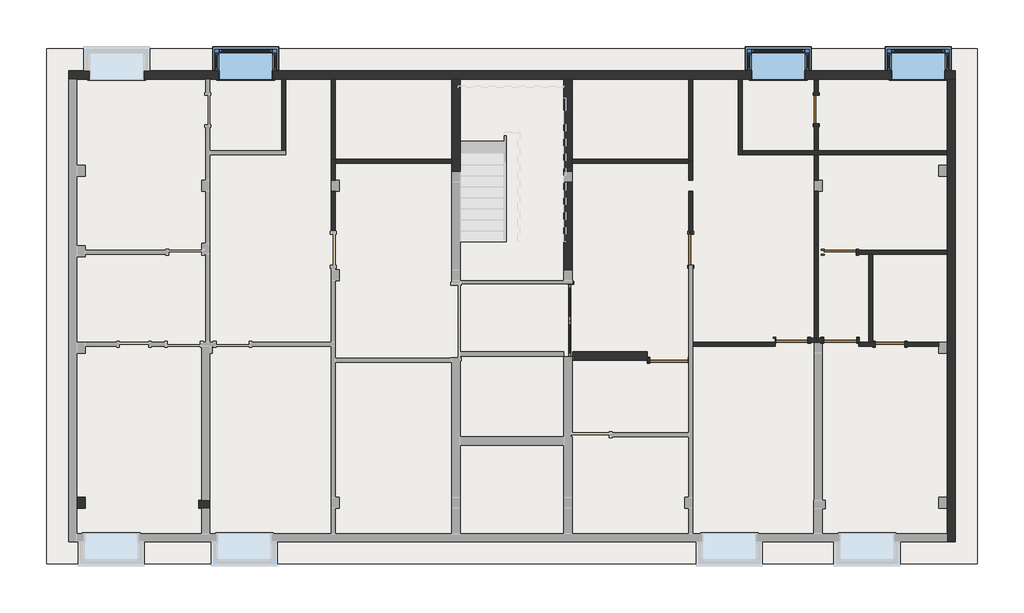
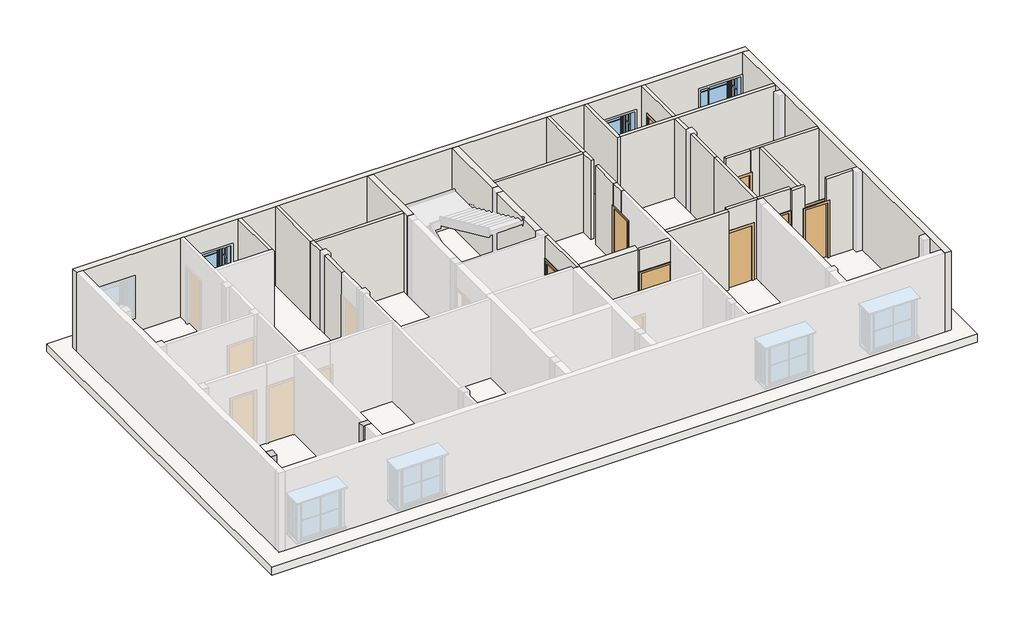
# One storey, part 2 of 3: 32 walls, 8 doors, 3 windows, 2 columns, 1 slab.
"""IFC4 building model written with IfcOpenShell, lengths in millimetres."""

from ifc_helpers import new_model, si_unit, frame, origin, place, context, project, spatial, polyline, outline, extrude, faceted_brep, transform, mapped, element, save
from components import door_04ab2522, m_door_single_panel_05506f71, door_85b31ab1, door_1991e9a2, door_a431d384, door_82def9da, m_door_single_panel_3_x7_f8176753, window_19bbd869

model = new_model("IFC4")

# Units and contexts
model_context = context("Model", 3, world=origin())
ifc_project = project(units=[si_unit("LENGTHUNIT", "METRE", prefix="MILLI")], contexts=[model_context])

# Site, building, storey
site = spatial("IfcSite", under=ifc_project)
building = spatial("IfcBuilding", under=site)
storey = spatial("IfcBuildingStorey", under=building, Elevation=12801.6)

# Columns
placement = place(None, origin())
element("IfcColumn", 1, ObjectType="Rectangular Column : 1'X 9\"", at=placement, inside=storey, context=model_context, shape_type="SweptSolid", body=[
    extrude(outline(polyline([(-12224.6987957, -3709.2932671), (-12224.6987957, -4014.0932671), (-12453.2987957, -4014.0932671), (-12453.2987957, -3709.2932671), (-12224.6987957, -3709.2932671)])), frame((0.0, 0.0, 12801.6), z_axis=(0.0, 0.0, 1.0), x_axis=(1.0, 0.0, 0.0)), (0.0, 0.0, 1.0), 3048.0),
])
element("IfcColumn", 2, ObjectType="Rectangular Column : 1'X 9\"", at=placement, inside=storey, context=model_context, shape_type="Brep", body=[
    faceted_brep([(-9076.550543, -3785.4932196, 12801.6), (-9000.350543, -3785.4932196, 12801.6), (-8771.750543, -3785.4932196, 12801.6), (-8771.750543, -4014.0932196, 12801.6), (-9000.350543, -4014.0932196, 12801.6), (-9076.550543, -4014.0932196, 12801.6), (-9076.550543, -3785.4932196, 15849.6), (-9000.350543, -3785.4932196, 15849.6), (-8771.750543, -3785.4932196, 15849.6), (-8771.750543, -4014.0932196, 15849.6), (-9000.350543, -4014.0932196, 15849.6), (-9076.550543, -4014.0932196, 15849.6)], [[[0, 1, 2, 3, 4, 5]], [[6, 7, 8, 2, 1, 0]], [[8, 9, 3, 2]], [[9, 10, 11, 5, 4, 3]], [[11, 6, 0, 5]], [[6, 11, 10, 9, 8, 7]]]),
])

# Doors
door_shape = door_04ab2522(model_context)
element("IfcDoor", 3, ObjectType="M_Door-Double-Glass : 6'7\"X7'", at=placement, inside=storey, context=model_context, shape_type="MappedRepresentation", body=[
    mapped(door_shape, transform((1217.5394962, 1183.3817656, 12801.6), x_axis=(0.0, 1.0, 0.0), y_axis=(-1.0, 0.0, 0.0), z_axis=(0.0, 0.0, 1.0))),
])
m_door_single_panel_shape = m_door_single_panel_05506f71(model_context)
element("IfcDoor", 4, ObjectType="M_Door-Single-Panel", at=placement, inside=storey, context=model_context, shape_type="MappedRepresentation", body=[
    mapped(m_door_single_panel_shape, transform((3933.4813133, 90.9578621, 12801.6), x_axis=(1.0, 0.0, 0.0), y_axis=(0.0, 1.0, 0.0), z_axis=(0.0, 0.0, 1.0))),
])
door_2_shape = door_85b31ab1(model_context)
element("IfcDoor", 5, ObjectType="M_Door-Single-Panel : 2'10\"X7' 2", at=placement, inside=storey, context=model_context, shape_type="MappedRepresentation", body=[
    mapped(door_2_shape, transform((4532.9512082, 3142.9626891, 12801.6), x_axis=(0.0, -1.0, 0.0), y_axis=(1.0, 0.0, 0.0), z_axis=(0.0, 0.0, 1.0))),
])
door_3_shape = door_1991e9a2(model_context)
element("IfcDoor", 6, ObjectType="M_Door-Single-Panel : 2'11\"X7' 3", at=placement, inside=storey, context=model_context, shape_type="MappedRepresentation", body=[
    mapped(door_3_shape, transform((7330.1405552, 640.4567334, 12801.6), x_axis=(1.0, 0.0, 0.0), y_axis=(0.0, 1.0, 0.0), z_axis=(0.0, 0.0, 1.0))),
])
element("IfcDoor", 7, ObjectType="M_Door-Single-Panel : 2'11\"X7' 3", at=placement, inside=storey, context=model_context, shape_type="MappedRepresentation", body=[
    mapped(door_3_shape, transform((8664.274939, 3078.8567332, 12801.6), x_axis=(-1.0, 0.0, 0.0), y_axis=(0.0, -1.0, 0.0), z_axis=(0.0, 0.0, 1.0))),
])
door_4_shape = door_a431d384(model_context)
element("IfcDoor", 8, ObjectType="M_Door-Single-Panel : 2'7\"X7' 2", at=placement, inside=storey, context=model_context, shape_type="MappedRepresentation", body=[
    mapped(door_4_shape, transform((8000.0512079, 7021.3751452, 12801.6), x_axis=(0.0, 1.0, 0.0), y_axis=(-1.0, 0.0, 0.0), z_axis=(0.0, 0.0, 1.0))),
])
door_5_shape = door_82def9da(model_context)
element("IfcDoor", 9, ObjectType="M_Door-Single-Panel : 2'8\"X7'", at=placement, inside=storey, context=model_context, shape_type="MappedRepresentation", body=[
    mapped(door_5_shape, transform((10046.0486694, 526.1567295, 12801.6), x_axis=(-1.0, 0.0, 0.0), y_axis=(0.0, -1.0, 0.0), z_axis=(0.0, 0.0, 1.0))),
])
m_door_single_panel_3_x7_shape = m_door_single_panel_3_x7_f8176753(model_context)
element("IfcDoor", 10, ObjectType="M_Door-Single-Panel : 3'X7'", at=placement, inside=storey, context=model_context, shape_type="MappedRepresentation", body=[
    mapped(m_door_single_panel_3_x7_shape, transform((8666.8012079, 640.4567334, 12801.6), x_axis=(-1.0, 0.0, 0.0), y_axis=(0.0, -1.0, 0.0), z_axis=(0.0, 0.0, 1.0))),
])

# Slab
element("IfcSlab", 11, ObjectType="Generic - 12\"", at=placement, inside=storey, context=model_context, shape_type="SweptSolid", body=[
    extrude(outline(polyline([(12464.1012075, 8698.6067329), (12464.1012075, -5550.7932662), (-13291.4987957, -5550.7932662), (-13291.4987957, 8698.6067329), (12464.1012075, 8698.6067329)])), frame((0.0, 0.0, 12496.8), z_axis=(0.0, 0.0, 1.0), x_axis=(1.0, 0.0, 0.0)), (0.0, 0.0, 1.0), 304.8),
])

# Walls
element("IfcWall", 12, ObjectType="4.5\"", at=placement, inside=storey, context=model_context, shape_type="SweptSolid", body=[
    extrude(outline(polyline([(3132.0737955, 15849.6), (3628.3344162, 15849.6), (3628.3344162, 12801.6), (3574.7626891, 12801.6), (3574.7626891, 14935.2), (3132.0737955, 14935.2), (3132.0737955, 15849.6)])), frame((4475.8012082, 0.0, 0.0), z_axis=(1.0, 0.0, 0.0), x_axis=(0.0, 1.0, 0.0)), (0.0, 0.0, 1.0), 114.3),
])
element("IfcWall", 13, ObjectType="4.5\"", at=placement, inside=storey, context=model_context, shape_type="Brep", body=[
    faceted_brep([(8000.0512079, 583.3067334, 12801.6), (8000.0512079, 583.3067334, 15849.6), (7942.9012047, 583.3067334, 15849.6), (6862.7668241, 583.3067334, 15849.6), (6862.7668241, 583.3067334, 12801.6), (6885.6405552, 583.3067334, 12801.6), (6885.6405552, 583.3067334, 14935.2), (7774.6405552, 583.3067334, 14935.2), (7774.6405552, 583.3067334, 12801.6), (7942.9012047, 583.3067334, 12801.6), (8000.0512079, 697.6067334, 15849.6), (8000.0512079, 697.6067334, 12801.6), (7942.9012079, 697.6067334, 12801.6), (7774.6405552, 697.6067334, 12801.6), (7774.6405552, 697.6067334, 14935.2), (6885.6405552, 697.6067334, 14935.2), (6885.6405552, 697.6067334, 12801.6), (6862.7668241, 697.6067334, 12801.6), (6862.7668241, 697.6067334, 15849.6), (7942.9012079, 697.6067334, 15849.6)], [[[0, 1, 2, 3, 4, 5, 6, 7, 8, 9]], [[10, 11, 12, 13, 14, 15, 16, 17, 18, 19]], [[4, 17, 16, 5]], [[11, 0, 9, 8, 13, 12]], [[1, 0, 11, 10]], [[3, 2, 1, 10, 19, 18]], [[4, 3, 18, 17]], [[7, 14, 13, 8]], [[14, 7, 6, 15]], [[15, 6, 5, 16]]]),
])
element("IfcWall", 14, ObjectType="4.5\"", at=placement, inside=storey, context=model_context, shape_type="Brep", body=[
    faceted_brep([(9187.5012047, 583.3067334, 12801.6), (9187.5012047, 583.3067334, 15849.6), (8171.5012047, 583.3067334, 15849.6), (8000.0512079, 583.3067334, 15849.6), (8000.0512079, 583.3067334, 12801.6), (8171.5012047, 583.3067334, 12801.6), (8209.6012079, 583.3067334, 12801.6), (8209.6012079, 583.3067334, 14935.2), (9124.0012079, 583.3067334, 14935.2), (9124.0012079, 583.3067334, 12801.6), (9187.5012047, 697.6067334, 15849.6), (9187.5012047, 697.6067334, 12801.6), (9124.0012079, 697.6067334, 12801.6), (9124.0012079, 697.6067334, 14935.2), (8209.6012079, 697.6067334, 14935.2), (8209.6012079, 697.6067334, 12801.6), (8057.2012079, 697.6067334, 12801.6), (8000.0512079, 697.6067334, 12801.6), (8000.0512079, 697.6067334, 15849.6), (8057.2012079, 697.6067334, 15849.6)], [[[0, 1, 2, 3, 4, 5, 6, 7, 8, 9]], [[10, 11, 12, 13, 14, 15, 16, 17, 18, 19]], [[11, 0, 9, 12]], [[4, 17, 16, 15, 6, 5]], [[1, 0, 11, 10]], [[3, 2, 1, 10, 19, 18]], [[4, 3, 18, 17]], [[7, 14, 13, 8]], [[8, 13, 12, 9]], [[14, 7, 6, 15]]]),
])
element("IfcWall", 15, ObjectType="4.5\"", at=placement, inside=storey, context=model_context, shape_type="SweptSolid", body=[
    extrude(outline(polyline([(12801.6, 9131.6486701), (15849.6, 9131.6486701), (15849.6, 8245.174939), (14935.2, 8245.174939), (14935.2, 9108.774939), (12801.6, 9108.774939), (12801.6, 9131.6486701)])), frame((0.0, 3021.7067332, 0.0), z_axis=(0.0, 1.0, 0.0), x_axis=(0.0, 0.0, 1.0)), (0.0, 0.0, 1.0), 114.3),
])
element("IfcWall", 16, ObjectType="4.5\"", at=placement, inside=storey, context=model_context, shape_type="SweptSolid", body=[
    extrude(outline(polyline([(5879.2067329, 15849.6), (7860.4067329, 15849.6), (7860.4067329, 12801.6), (7415.0751452, 12801.6), (7415.0751452, 14935.2), (6627.6751452, 14935.2), (6627.6751452, 12801.6), (5879.2067329, 12801.6), (5879.2067329, 15849.6)])), frame((7942.9012079, 0.0, 0.0), z_axis=(1.0, 0.0, 0.0), x_axis=(0.0, 1.0, 0.0)), (0.0, 0.0, 1.0), 114.3),
])
element("IfcWall", 17, ObjectType="4.5\"", at=placement, inside=storey, context=model_context, shape_type="Brep", body=[
    faceted_brep([(4466.8813133, 33.8078621, 14935.2), (4466.8813133, 33.8078621, 12801.6), (4475.8012082, 33.8078621, 12801.6), (4475.8012082, 33.8078621, 15849.6), (3334.0114184, 33.8078621, 15849.6), (3334.0114184, 33.8078621, 12801.6), (3400.0813133, 33.8078621, 12801.6), (3400.0813133, 33.8078621, 14935.2), (4475.8012082, 148.1078621, 12801.6), (4466.8813133, 148.1078621, 12801.6), (4466.8813133, 148.1078621, 14935.2), (3400.0813133, 148.1078621, 14935.2), (3400.0813133, 148.1078621, 12801.6), (3334.0114184, 148.1078621, 12801.6), (3334.0114184, 148.1078621, 15849.6), (4475.8012082, 148.1078621, 15849.6), (3334.0114184, 90.9578621, 12801.6), (3334.0114184, 90.9578621, 15849.6)], [[[0, 1, 2, 3, 4, 5, 6, 7]], [[8, 9, 10, 11, 12, 13, 14, 15]], [[6, 5, 16, 13, 12]], [[2, 1, 9, 8]], [[4, 3, 15, 14, 17]], [[5, 4, 17, 14, 13, 16]], [[3, 2, 8, 15]], [[10, 9, 1, 0]], [[11, 10, 0, 7]], [[12, 11, 7, 6]]]),
])
element("IfcWall", 18, ObjectType="4.5\"", at=placement, inside=storey, context=model_context, shape_type="Brep", body=[
    faceted_brep([(1158.0082462, 205.2578621, 15849.6), (1158.0082462, 2196.2067742, 15849.6), (1158.0082462, 2196.2067742, 12801.6), (1158.0082462, 2186.6817656, 12801.6), (1158.0082462, 2186.6817656, 14935.2), (1158.0082462, 205.2578621, 14935.2), (1272.3082462, 2196.2067742, 15849.6), (1272.3082462, 319.5578621, 15849.6), (1272.3082462, 205.2578621, 15849.6), (1272.3082462, 205.2578621, 14935.2), (1272.3082462, 2186.6817656, 14935.2), (1272.3082462, 2186.6817656, 12801.6), (1272.3082462, 2196.2067742, 12801.6), (1250.0012085, 205.2578621, 15849.6), (1250.0012085, 205.2578621, 14935.2)], [[[0, 1, 2, 3, 4, 5]], [[6, 7, 8, 9, 10, 11, 12]], [[2, 12, 11, 3]], [[8, 13, 0, 5, 14, 9]], [[1, 0, 13, 8, 7, 6]], [[2, 1, 6, 12]], [[10, 4, 3, 11]], [[4, 10, 9, 14, 5]]]),
])
element("IfcWall", 19, ObjectType="4.5\"", at=placement, inside=storey, context=model_context, shape_type="Brep", body=[
    faceted_brep([(1250.0012085, 5536.3067329, 12801.6), (4475.8012082, 5536.3067329, 12801.6), (4475.8012082, 5536.3067329, 15849.6), (1250.0012085, 5536.3067329, 15849.6), (1250.0012085, 5650.6067329, 12801.6), (1250.0012085, 5650.6067329, 15849.6), (4475.8012082, 5650.6067329, 15849.6), (4475.8012082, 5650.6067329, 12801.6), (4475.8012082, 5593.4567329, 12801.6), (4475.8012082, 5593.4567329, 15849.6)], [[[0, 1, 2, 3]], [[4, 5, 6, 7]], [[1, 0, 4, 7, 8]], [[3, 2, 9, 6, 5]], [[2, 1, 8, 7, 6, 9]], [[0, 3, 5, 4]]]),
])
element("IfcWall", 20, ObjectType="4.5\"", at=placement, inside=storey, context=model_context, shape_type="Brep", body=[
    faceted_brep([(8057.2012047, 3270.1432417, 12801.6), (8057.2012047, 4760.6824989, 12801.6), (8057.2012047, 4760.6824989, 15849.6), (8057.2012047, 3270.1432417, 15849.6), (7942.9012047, 3270.1432417, 12801.6), (7942.9012047, 3270.1432417, 15849.6), (7942.9012047, 4760.6824989, 15849.6), (7942.9012047, 4760.6824989, 12801.6), (7943.9040565, 4760.6824989, 12801.6), (7943.9040565, 4760.6824989, 15849.6)], [[[0, 1, 2, 3]], [[4, 5, 6, 7]], [[1, 0, 4, 7, 8]], [[2, 1, 8, 7, 6, 9]], [[3, 2, 9, 6, 5]], [[0, 3, 5, 4]]]),
])
element("IfcWall", 21, ObjectType="4.5\"", at=placement, inside=storey, context=model_context, shape_type="Brep", body=[
    faceted_brep([(7942.9012079, 3270.1432417, 12801.6), (7942.9012079, 697.6067334, 12801.6), (7942.9012079, 697.6067334, 15849.6), (7942.9012079, 3270.1432417, 15849.6), (8057.2012079, 3270.1432417, 12801.6), (8057.2012079, 3270.1432417, 15849.6), (8057.2012079, 697.6067334, 15849.6), (8057.2012079, 697.6067334, 12801.6), (8000.0512079, 697.6067334, 12801.6), (8000.0512079, 697.6067334, 15849.6)], [[[0, 1, 2, 3]], [[4, 5, 6, 7]], [[1, 0, 4, 7, 8]], [[3, 2, 9, 6, 5]], [[0, 3, 5, 4]], [[2, 1, 8, 7, 6, 9]]]),
])
element("IfcWall", 22, ObjectType="4.5\"", at=placement, inside=storey, context=model_context, shape_type="SweptSolid", body=[
    extrude(outline(polyline([(8058.2040565, 5763.9824989), (8058.2040565, 5065.4824989), (7943.9040565, 5065.4824989), (7943.9040565, 5763.9824989), (8058.2040565, 5763.9824989)])), frame((0.0, 0.0, 12801.6), z_axis=(0.0, 0.0, 1.0), x_axis=(1.0, 0.0, 0.0)), (0.0, 0.0, 1.0), 3048.0),
])
element("IfcWall", 23, ObjectType="4.5\" 2", at=placement, inside=storey, context=model_context, shape_type="SweptSolid", body=[
    extrude(outline(polyline([(-6674.7987994, 7860.4067329), (-6674.7987994, 5879.2067329), (-6789.0987994, 5879.2067329), (-6789.0987994, 7860.4067329), (-6674.7987994, 7860.4067329)])), frame((0.0, 0.0, 12801.6), z_axis=(0.0, 0.0, 1.0), x_axis=(1.0, 0.0, 0.0)), (0.0, 0.0, 1.0), 3048.0),
])
element("IfcWall", 24, ObjectType="4.5\" 2", at=placement, inside=storey, context=model_context, shape_type="SweptSolid", body=[
    extrude(outline(polyline([(-5303.1987995, 4761.606733), (-5303.1987995, 3671.8272228), (-5417.4987995, 3671.8272228), (-5417.4987995, 4761.606733), (-5303.1987995, 4761.606733)])), frame((0.0, 0.0, 12801.6), z_axis=(0.0, 0.0, 1.0), x_axis=(1.0, 0.0, 0.0)), (0.0, 0.0, 1.0), 3048.0),
])
element("IfcWall", 25, ObjectType="4.5\" 2", at=placement, inside=storey, context=model_context, shape_type="Brep", body=[
    faceted_brep([(-5303.1987995, 5066.406733, 12801.6), (-5303.1987995, 5536.3067329, 12801.6), (-5303.1987995, 5650.6067329, 12801.6), (-5303.1987995, 5650.6067329, 15849.6), (-5303.1987995, 5536.3067329, 15849.6), (-5303.1987995, 5066.406733, 15849.6), (-5417.4987995, 5066.406733, 12801.6), (-5417.4987995, 5066.406733, 15849.6), (-5417.4987995, 5650.6067329, 15849.6), (-5417.4987995, 5650.6067329, 12801.6)], [[[0, 1, 2, 3, 4, 5]], [[6, 7, 8, 9]], [[2, 1, 0, 6, 9]], [[5, 4, 3, 8, 7]], [[0, 5, 7, 6]], [[3, 2, 9, 8]]]),
])
element("IfcWall", 26, ObjectType="4.5\" 2", at=placement, inside=storey, context=model_context, shape_type="SweptSolid", body=[
    extrude(outline(polyline([(-2077.3987998, 5536.3067329), (-5303.1987995, 5536.3067329), (-5303.1987995, 5650.6067329), (-2077.3987998, 5650.6067329), (-2077.3987998, 5536.3067329)])), frame((0.0, 0.0, 12801.6), z_axis=(0.0, 0.0, 1.0), x_axis=(1.0, 0.0, 0.0)), (0.0, 0.0, 1.0), 3048.0),
])
element("IfcWall", 27, ObjectType="4.5\" 2", at=placement, inside=storey, context=model_context, shape_type="SweptSolid", body=[
    extrude(outline(polyline([(-5417.4987995, 5650.6067329), (-5417.4987995, 7860.4067329), (-5303.1987995, 7860.4067329), (-5303.1987995, 5650.6067329), (-5417.4987995, 5650.6067329)])), frame((0.0, 0.0, 12801.6), z_axis=(0.0, 0.0, 1.0), x_axis=(1.0, 0.0, 0.0)), (0.0, 0.0, 1.0), 3048.0),
])
element("IfcWall", 28, ObjectType="4.5\" 2", at=placement, inside=storey, context=model_context, shape_type="Brep", body=[
    faceted_brep([(4475.8012082, 5593.4567329, 12801.6), (4475.8012082, 5536.3067329, 12801.6), (4475.8012082, 5066.40678, 12801.6), (4475.8012082, 5066.40678, 15849.6), (4475.8012082, 5536.3067329, 15849.6), (4475.8012082, 5593.4567329, 15849.6), (4590.1012082, 5593.4567329, 12801.6), (4590.1012082, 5593.4567329, 15849.6), (4590.1012082, 5066.40678, 15849.6), (4590.1012082, 5066.40678, 12801.6)], [[[0, 1, 2, 3, 4, 5]], [[6, 7, 8, 9]], [[2, 1, 0, 6, 9]], [[3, 2, 9, 8]], [[5, 4, 3, 8, 7]], [[0, 5, 7, 6]]]),
])
element("IfcWall", 29, ObjectType="4.5\" 2", at=placement, inside=storey, context=model_context, shape_type="SweptSolid", body=[
    extrude(outline(polyline([(4475.8012082, 3628.3344162), (4475.8012082, 4761.606733), (4590.1012082, 4761.606733), (4590.1012082, 3628.3344162), (4475.8012082, 3628.3344162)])), frame((0.0, 0.0, 12801.6), z_axis=(0.0, 0.0, 1.0), x_axis=(1.0, 0.0, 0.0)), (0.0, 0.0, 1.0), 3048.0),
])
element("IfcWall", 30, ObjectType="4.5\" 2", at=placement, inside=storey, context=model_context, shape_type="SweptSolid", body=[
    extrude(outline(polyline([(6862.7668241, 469.0067334), (4590.1012082, 469.0067334), (4590.1012082, 583.3067334), (6862.7668241, 583.3067334), (6862.7668241, 469.0067334)])), frame((0.0, 0.0, 12801.6), z_axis=(0.0, 0.0, 1.0), x_axis=(1.0, 0.0, 0.0)), (0.0, 0.0, 1.0), 3048.0),
])
element("IfcWall", 31, ObjectType="4.5\" 2", at=placement, inside=storey, context=model_context, shape_type="Brep", body=[
    faceted_brep([(9182.4486694, 469.0067295, 12801.6), (9639.6486694, 469.0067295, 12801.6), (9639.6486694, 469.0067295, 15849.6), (9182.4486694, 469.0067295, 15849.6), (9182.4486694, 583.3067295, 12801.6), (9182.4486694, 583.3067295, 15849.6), (9451.1098918, 583.3067295, 15849.6), (9565.4098918, 583.3067295, 15849.6), (9639.6486694, 583.3067295, 15849.6), (9639.6486694, 583.3067295, 12801.6), (9565.4098918, 583.3067295, 12801.6), (9451.1098918, 583.3067295, 12801.6)], [[[0, 1, 2, 3]], [[4, 5, 6, 7, 8, 9, 10, 11]], [[1, 0, 4, 11, 10, 9]], [[2, 1, 9, 8]], [[3, 2, 8, 7, 6, 5]], [[0, 3, 5, 4]]]),
])
element("IfcWall", 32, ObjectType="4.5\" 2", at=placement, inside=storey, context=model_context, shape_type="SweptSolid", body=[
    extrude(outline(polyline([(12801.6, 11397.3012075), (15849.6, 11397.3012075), (15849.6, 10443.8236977), (14935.2, 10443.8236977), (14935.2, 10452.4486694), (12801.6, 10452.4486694), (12801.6, 11397.3012075)])), frame((0.0, 469.0067295, 0.0), z_axis=(0.0, 1.0, 0.0), x_axis=(0.0, 0.0, 1.0)), (0.0, 0.0, 1.0), 114.3),
])
element("IfcWall", 33, ObjectType="4.5\" 2", at=placement, inside=storey, context=model_context, shape_type="SweptSolid", body=[
    extrude(outline(polyline([(9565.4098918, 3021.7067332), (9565.4098918, 583.3067295), (9451.1098918, 583.3067295), (9451.1098918, 3021.7067332), (9565.4098918, 3021.7067332)])), frame((0.0, 0.0, 12801.6), z_axis=(0.0, 0.0, 1.0), x_axis=(1.0, 0.0, 0.0)), (0.0, 0.0, 1.0), 3048.0),
])
element("IfcWall", 34, ObjectType="4.5\" 2", at=placement, inside=storey, context=model_context, shape_type="Brep", body=[
    faceted_brep([(9131.6486701, 3021.7067332, 12801.6), (9451.1098918, 3021.7067332, 12801.6), (9565.4098918, 3021.7067332, 12801.6), (11625.9012075, 3021.7067332, 12801.6), (11625.9012075, 3021.7067332, 15849.6), (9565.4098918, 3021.7067332, 15849.6), (9451.1098918, 3021.7067332, 15849.6), (9131.6486701, 3021.7067332, 15849.6), (9131.6486701, 3136.0067332, 12801.6), (9131.6486701, 3136.0067332, 15849.6), (11625.9012075, 3136.0067332, 15849.6), (11625.9012075, 3136.0067332, 12801.6)], [[[0, 1, 2, 3, 4, 5, 6, 7]], [[8, 9, 10, 11]], [[3, 2, 1, 0, 8, 11]], [[7, 6, 5, 4, 10, 9]], [[0, 7, 9, 8]], [[4, 3, 11, 10]]]),
])
element("IfcWall", 35, ObjectType="4.5\" 2", at=placement, inside=storey, context=model_context, shape_type="Brep", body=[
    faceted_brep([(4590.1012082, 5593.4567329, 12801.6), (4590.1012082, 7860.4067329, 12801.6), (4590.1012082, 7860.4067329, 15849.6), (4590.1012082, 5593.4567329, 15849.6), (4475.8012082, 5593.4567329, 12801.6), (4475.8012082, 5593.4567329, 15849.6), (4475.8012082, 5650.6067329, 15849.6), (4475.8012082, 7860.4067329, 15849.6), (4475.8012082, 7860.4067329, 12801.6), (4475.8012082, 5650.6067329, 12801.6)], [[[0, 1, 2, 3]], [[4, 5, 6, 7, 8, 9]], [[1, 0, 4, 9, 8]], [[3, 2, 7, 6, 5]], [[0, 3, 5, 4]], [[2, 1, 8, 7]]]),
])
element("IfcWall", 36, ObjectType="4.5\" 2", at=placement, inside=storey, context=model_context, shape_type="Brep", body=[
    faceted_brep([(5847.401208, 7860.4067329, 12801.6), (5847.401208, 5764.9067329, 12801.6), (5847.401208, 5764.9067329, 15849.6), (5847.401208, 7860.4067329, 15849.6), (5961.701208, 7860.4067329, 12801.6), (5961.701208, 7860.4067329, 15849.6), (5961.701208, 5879.2067329, 15849.6), (5961.701208, 5764.9067329, 15849.6), (5961.701208, 5764.9067329, 12801.6), (5961.701208, 5879.2067329, 12801.6)], [[[0, 1, 2, 3]], [[4, 5, 6, 7, 8, 9]], [[1, 0, 4, 9, 8]], [[3, 2, 7, 6, 5]], [[2, 1, 8, 7]], [[0, 3, 5, 4]]]),
])
element("IfcWall", 37, ObjectType="4.5\" 2", at=placement, inside=storey, context=model_context, shape_type="Brep", body=[
    faceted_brep([(5961.701208, 5764.9067329, 12801.6), (11625.9012075, 5764.9067329, 12801.6), (11625.9012075, 5764.9067329, 15849.6), (5961.701208, 5764.9067329, 15849.6), (5961.701208, 5879.2067329, 12801.6), (5961.701208, 5879.2067329, 15849.6), (7942.9012079, 5879.2067329, 15849.6), (8057.2012079, 5879.2067329, 15849.6), (11625.9012075, 5879.2067329, 15849.6), (11625.9012075, 5879.2067329, 12801.6), (8057.2012079, 5879.2067329, 12801.6), (7942.9012079, 5879.2067329, 12801.6)], [[[0, 1, 2, 3]], [[4, 5, 6, 7, 8, 9, 10, 11]], [[1, 0, 4, 11, 10, 9]], [[3, 2, 8, 7, 6, 5]], [[0, 3, 5, 4]], [[2, 1, 9, 8]]]),
])
element("IfcWall", 38, ObjectType="9\"", at=placement, inside=storey, context=model_context, shape_type="Brep", body=[
    faceted_brep([(-12681.8987957, 7860.4067329, 12801.6), (-12453.2987957, 7860.4067329, 12801.6), (-8884.5987992, 7860.4067329, 12801.6), (-8770.2987992, 7860.4067329, 12801.6), (-6789.0987994, 7860.4067329, 12801.6), (-6674.7987994, 7860.4067329, 12801.6), (-5417.4987995, 7860.4067329, 12801.6), (-5303.1987995, 7860.4067329, 12801.6), (-2074.1417538, 7860.4067329, 12801.6), (-1845.5417538, 7860.4067329, 12801.6), (1021.4012085, 7860.4067329, 12801.6), (1250.0012085, 7860.4067329, 12801.6), (4475.8012082, 7860.4067329, 12801.6), (4590.1012082, 7860.4067329, 12801.6), (5847.401208, 7860.4067329, 12801.6), (5961.701208, 7860.4067329, 12801.6), (7942.9012079, 7860.4067329, 12801.6), (8057.2012079, 7860.4067329, 12801.6), (11625.9012075, 7860.4067329, 12801.6), (11854.5012075, 7860.4067329, 12801.6), (11854.5012075, 7860.4067329, 15849.6), (11625.9012075, 7860.4067329, 15849.6), (8057.2012079, 7860.4067329, 15849.6), (7942.9012079, 7860.4067329, 15849.6), (5961.701208, 7860.4067329, 15849.6), (5847.401208, 7860.4067329, 15849.6), (4590.1012082, 7860.4067329, 15849.6), (4475.8012082, 7860.4067329, 15849.6), (1250.0012085, 7860.4067329, 15849.6), (1021.4012085, 7860.4067329, 15849.6), (-1845.5417538, 7860.4067329, 15849.6), (-2074.1417538, 7860.4067329, 15849.6), (-5303.1987995, 7860.4067329, 15849.6), (-5417.4987995, 7860.4067329, 15849.6), (-6674.7987994, 7860.4067329, 15849.6), (-6789.0987994, 7860.4067329, 15849.6), (-8770.2987992, 7860.4067329, 15849.6), (-8884.5987992, 7860.4067329, 15849.6), (-12453.2987957, 7860.4067329, 15849.6), (-12681.8987957, 7860.4067329, 15849.6), (11575.8012075, 7860.4067329, 14952.4), (11575.8012075, 7860.4067329, 13401.6), (10075.8012075, 7860.4067329, 13401.6), (10075.8012075, 7860.4067329, 14952.4), (7702.301208, 7860.4067329, 14952.4), (7702.301208, 7860.4067329, 13401.6), (6202.301208, 7860.4067329, 13401.6), (6202.301208, 7860.4067329, 14952.4), (-7029.6987993, 7860.4067329, 14952.4), (-7029.6987993, 7860.4067329, 13401.6), (-8529.6987993, 7860.4067329, 13401.6), (-8529.6987993, 7860.4067329, 14952.4), (-10598.3987957, 7860.4067329, 14952.4), (-10598.3987957, 7860.4067329, 13401.6), (-12098.3987957, 7860.4067329, 13401.6), (-12098.3987957, 7860.4067329, 14952.4), (-12681.8987957, 8089.0067329, 12801.6), (-12681.8987957, 8089.0067329, 15849.6), (11854.5012075, 8089.0067329, 15849.6), (11854.5012075, 8089.0067329, 12801.6), (11575.8012075, 8089.0067329, 14952.4), (10075.8012075, 8089.0067329, 14952.4), (10075.8012075, 8089.0067329, 13401.6), (11575.8012075, 8089.0067329, 13401.6), (7702.301208, 8089.0067329, 14952.4), (6202.301208, 8089.0067329, 14952.4), (6202.301208, 8089.0067329, 13401.6), (7702.301208, 8089.0067329, 13401.6), (-7029.6987993, 8089.0067329, 14952.4), (-8529.6987993, 8089.0067329, 14952.4), (-8529.6987993, 8089.0067329, 13401.6), (-7029.6987993, 8089.0067329, 13401.6), (-10598.3987957, 8089.0067329, 14952.4), (-12098.3987957, 8089.0067329, 14952.4), (-12098.3987957, 8089.0067329, 13401.6), (-10598.3987957, 8089.0067329, 13401.6)], [[[0, 1, 2, 3, 4, 5, 6, 7, 8, 9, 10, 11, 12, 13, 14, 15, 16, 17, 18, 19, 20, 21, 22, 23, 24, 25, 26, 27, 28, 29, 30, 31, 32, 33, 34, 35, 36, 37, 38, 39], [40, 41, 42, 43], [44, 45, 46, 47], [48, 49, 50, 51], [52, 53, 54, 55]], [[56, 57, 58, 59], [60, 61, 62, 63], [64, 65, 66, 67], [68, 69, 70, 71], [72, 73, 74, 75]], [[19, 18, 17, 16, 15, 14, 13, 12, 11, 10, 9, 8, 7, 6, 5, 4, 3, 2, 1, 0, 56, 59]], [[39, 38, 37, 36, 35, 34, 33, 32, 31, 30, 29, 28, 27, 26, 25, 24, 23, 22, 21, 20, 58, 57]], [[20, 19, 59, 58]], [[0, 39, 57, 56]], [[41, 40, 60, 63]], [[42, 41, 63, 62]], [[43, 42, 62, 61]], [[40, 43, 61, 60]], [[45, 44, 64, 67]], [[46, 45, 67, 66]], [[47, 46, 66, 65]], [[44, 47, 65, 64]], [[49, 48, 68, 71]], [[50, 49, 71, 70]], [[51, 50, 70, 69]], [[48, 51, 69, 68]], [[53, 52, 72, 75]], [[54, 53, 75, 74]], [[55, 54, 74, 73]], [[52, 55, 73, 72]]]),
])
element("IfcWall", 39, ObjectType="9\"", at=placement, inside=storey, context=model_context, shape_type="Brep", body=[
    faceted_brep([(11625.9012075, 7860.4067329, 12801.6), (11625.9012075, 5879.2067329, 12801.6), (11625.9012075, 5764.9067329, 12801.6), (11625.9012075, 5479.1567329, 12801.6), (11625.9012075, 5174.3567329, 12801.6), (11625.9012075, 3136.0067332, 12801.6), (11625.9012075, 3021.7067332, 12801.6), (11625.9012075, 583.3067295, 12801.6), (11625.9012075, 278.5067295, 12801.6), (11625.9012075, -3709.2932671, 12801.6), (11625.9012075, -4014.0932671, 12801.6), (11625.9012075, -4712.5932662, 12801.6), (11625.9012075, -4941.1932662, 12801.6), (11625.9012075, -4941.1932662, 15849.6), (11625.9012075, -4712.5932662, 15849.6), (11625.9012075, -4014.0932671, 15849.6), (11625.9012075, -3709.2932671, 15849.6), (11625.9012075, 278.5067295, 15849.6), (11625.9012075, 583.3067295, 15849.6), (11625.9012075, 3021.7067332, 15849.6), (11625.9012075, 3136.0067332, 15849.6), (11625.9012075, 5174.3567329, 15849.6), (11625.9012075, 5479.1567329, 15849.6), (11625.9012075, 5764.9067329, 15849.6), (11625.9012075, 5879.2067329, 15849.6), (11625.9012075, 7860.4067329, 15849.6), (11854.5012075, 7860.4067329, 12801.6), (11854.5012075, 7860.4067329, 15849.6), (11854.5012075, -4941.1932662, 15849.6), (11854.5012075, -4941.1932662, 12801.6)], [[[0, 1, 2, 3, 4, 5, 6, 7, 8, 9, 10, 11, 12, 13, 14, 15, 16, 17, 18, 19, 20, 21, 22, 23, 24, 25]], [[26, 27, 28, 29]], [[12, 11, 10, 9, 8, 7, 6, 5, 4, 3, 2, 1, 0, 26, 29]], [[25, 24, 23, 22, 21, 20, 19, 18, 17, 16, 15, 14, 13, 28, 27]], [[0, 25, 27, 26]], [[13, 12, 29, 28]]]),
])
element("IfcWall", 40, ObjectType="9\"", at=placement, inside=storey, context=model_context, shape_type="SweptSolid", body=[
    extrude(outline(polyline([(-2074.1417538, 5320.4067329), (-2074.1417538, 7860.4067329), (-1845.5417538, 7860.4067329), (-1845.5417538, 5320.4067329), (-2074.1417538, 5320.4067329)])), frame((0.0, 0.0, 12801.6), z_axis=(0.0, 0.0, 1.0), x_axis=(1.0, 0.0, 0.0)), (0.0, 0.0, 1.0), 3048.0),
])
element("IfcWall", 41, ObjectType="9\"", at=placement, inside=storey, context=model_context, shape_type="Brep", body=[
    faceted_brep([(1021.4012085, 7860.4067329, 12801.6), (1021.4012085, 5320.4067329, 12801.6), (1021.4012085, 5320.4067329, 15849.6), (1021.4012085, 7860.4067329, 15849.6), (1250.0012085, 7860.4067329, 12801.6), (1250.0012085, 7860.4067329, 15849.6), (1250.0012085, 5650.6067329, 15849.6), (1250.0012085, 5536.3067329, 15849.6), (1250.0012085, 5320.4067329, 15849.6), (1250.0012085, 5320.4067329, 12801.6), (1250.0012085, 5536.3067329, 12801.6), (1250.0012085, 5650.6067329, 12801.6)], [[[0, 1, 2, 3]], [[4, 5, 6, 7, 8, 9, 10, 11]], [[1, 0, 4, 11, 10, 9]], [[2, 1, 9, 8]], [[3, 2, 8, 7, 6, 5]], [[0, 3, 5, 4]]]),
])
element("IfcWall", 42, ObjectType="9\"", at=placement, inside=storey, context=model_context, shape_type="Brep", body=[
    faceted_brep([(1021.4012085, 5015.6067329, 12801.6), (1021.4012085, 2589.9067742, 12801.6), (1021.4012085, 2589.9067742, 15849.6), (1021.4012085, 5015.6067329, 15849.6), (1250.0012085, 5015.6067329, 12801.6), (1250.0012085, 5015.6067329, 15849.6), (1250.0012085, 2589.9067742, 15849.6), (1250.0012085, 2589.9067742, 12801.6), (1024.6582462, 2589.9067742, 12801.6), (1024.6582462, 2589.9067742, 15849.6)], [[[0, 1, 2, 3]], [[4, 5, 6, 7]], [[1, 0, 4, 7, 8]], [[2, 1, 8, 7, 6, 9]], [[3, 2, 9, 6, 5]], [[0, 3, 5, 4]]]),
])
element("IfcWall", 43, ObjectType="9\"", at=placement, inside=storey, context=model_context, shape_type="Brep", body=[
    faceted_brep([(3334.0114184, 319.5578621, 12801.6), (1272.3082462, 319.5578621, 12801.6), (1272.3082462, 319.5578621, 15849.6), (3334.0114184, 319.5578621, 15849.6), (1250.0012085, 90.9578621, 12801.6), (3334.0114184, 90.9578621, 12801.6), (3334.0114184, 90.9578621, 15849.6), (1250.0012085, 90.9578621, 15849.6), (1272.3082462, 180.0817656, 12801.6), (3334.0114184, 148.1078621, 12801.6), (1250.0012085, 180.0817656, 12801.6), (1272.3082462, 205.2578621, 15849.6), (1250.0012085, 205.2578621, 15849.6), (3334.0114184, 148.1078621, 15849.6), (1272.3082462, 180.0817656, 14935.2), (1272.3082462, 205.2578621, 14935.2), (1250.0012085, 205.2578621, 14935.2), (1250.0012085, 180.0817656, 14935.2)], [[[0, 1, 2, 3]], [[4, 5, 6, 7]], [[8, 1, 0, 9, 5, 4, 10]], [[3, 2, 11, 12, 7, 6, 13]], [[0, 3, 13, 6, 5, 9]], [[8, 14, 15, 11, 2, 1]], [[12, 11, 15, 16]], [[4, 7, 12, 16, 17, 10]], [[15, 14, 17, 16]], [[14, 8, 10, 17]]]),
])

# Windows
window_shape = window_19bbd869(model_context)
element("IfcWindow", 44, ObjectType="4'.8\"x3'.8\"", at=placement, inside=storey, context=model_context, shape_type="MappedRepresentation", body=[
    mapped(window_shape, transform((-7779.6987993, 7974.7067329, 12801.6), x_axis=(1.0, 0.0, 0.0), y_axis=(0.0, 1.0, 0.0), z_axis=(0.0, 0.0, 1.0))),
])
element("IfcWindow", 45, ObjectType="4'.8\"x3'.8\"", at=placement, inside=storey, context=model_context, shape_type="MappedRepresentation", body=[
    mapped(window_shape, transform((6952.301208, 7974.7067329, 12801.6), x_axis=(1.0, 0.0, 0.0), y_axis=(0.0, 1.0, 0.0), z_axis=(0.0, 0.0, 1.0))),
])
element("IfcWindow", 46, ObjectType="4'.8\"x3'.8\"", at=placement, inside=storey, context=model_context, shape_type="MappedRepresentation", body=[
    mapped(window_shape, transform((10825.8012075, 7974.7067329, 12801.6), x_axis=(1.0, 0.0, 0.0), y_axis=(0.0, 1.0, 0.0), z_axis=(0.0, 0.0, 1.0))),
])

save(model, "model.ifc")

# Revit data of these elements
# Type "Rectangular Column : 1'X 9\""
#   Assembly Code = "B1010200"
#   Depth = 1' - 0"
#   Offset Base = 0' - 0"
#   Offset Top = 0' - 0"
#   Width = 0' - 9"
#   Material = none
# Type "M_Door-Double-Glass : 6'7\"X7'"
#   Type Mark = "16"
#   Construction Type Id = "opn-d45"
#   Assembly Code = "C1020"
#   Analytic Construction = "Wood frame, double glass door "
#   W = 3' - 3 1/2"
#   Thickness = 0' - 1.9685"
#   Thermal Resistance (R) = 1.8150 (h·ft²·°F)/BTU
#   Swing Angle [instance default] = 90.00°
#   Heat Transfer Coefficient (U) = 0.5510 BTU/(h·ft²·°F)
#   Height = 7' - 0"
#   Bottom Rail = 0' - 3.93701"
#   Top Rail = 0' - 3.93701"
#   Stiles = 0' - 3.93701"
#   Trim Projection = 0' - 0.98425"
#   Trim Width = 0' - 3.14961"
#   Width = 6' - 7"
#   Define Thermal Properties by = 1
#   Glazing = Glass
#   Panel Material = Wood - Birch - Solid Stained Light Low Gloss
#   Trim Material = Paint - Sienna
#   Visual Light Transmittance = 0
#   Solar Heat Gain Coefficient = 0
#   Function = (empty or 0)
#   Wall Closure = (empty or 0)
# Type "M_Door-Single-Panel"
#   Type Mark = "14"
#   Construction Type Id = "DOOR"
#   Assembly Code = "C1020300"
#   Analytic Construction = "Wooden"
#   Thickness = 0' - 1.9685"
#   Thermal Resistance (R) = 2.5876 (h·ft²·°F)/BTU
#   Swing Angle [instance default] = 90.00°
#   Heat Transfer Coefficient (U) = 0.3865 BTU/(h·ft²·°F)
#   Height = 7' - 0"
#   Trim Projection Ext = 0' - 0.98425"
#   Trim Projection Int = 0' - 0.98425"
#   Trim Width = 0' - 3.14961"
#   Width = 3' - 6"
#   Define Thermal Properties by = 1
#   Panel Material = Wood - Birch - Solid Stained Light Low Gloss
#   Trim Material = Paint - Sienna
#   Visual Light Transmittance = 0
#   Solar Heat Gain Coefficient = 0
#   Function = (empty or 0)
#   Wall Closure = (empty or 0)
# Type "M_Door-Single-Panel : 2'10\"X7' 2"
#   Type Mark = "10"
#   Construction Type Id = "DOOR"
#   Assembly Code = "C1020300"
#   Analytic Construction = "Wooden"
#   Thickness = 0' - 1.9685"
#   Thermal Resistance (R) = 2.5876 (h·ft²·°F)/BTU
#   Swing Angle [instance default] = 90.00°
#   Heat Transfer Coefficient (U) = 0.3865 BTU/(h·ft²·°F)
#   Height = 7' - 0"
#   Trim Projection Ext = 0' - 0.98425"
#   Trim Projection Int = 0' - 0.98425"
#   Trim Width = 0' - 3.14961"
#   Width = 2' - 10"
#   Define Thermal Properties by = 1
#   Panel Material = Wood - Birch - Solid Stained Light Low Gloss
#   Trim Material = Paint - Sienna
#   Visual Light Transmittance = 0
#   Solar Heat Gain Coefficient = 0
#   Function = (empty or 0)
#   Wall Closure = (empty or 0)
# Type "M_Door-Single-Panel : 2'11\"X7' 3"
#   Type Mark = "12"
#   Construction Type Id = "DOOR"
#   Assembly Code = "C1020300"
#   Analytic Construction = "Wooden"
#   Thickness = 0' - 1.9685"
#   Thermal Resistance (R) = 2.5876 (h·ft²·°F)/BTU
#   Swing Angle [instance default] = 90.00°
#   Heat Transfer Coefficient (U) = 0.3865 BTU/(h·ft²·°F)
#   Height = 7' - 0"
#   Trim Projection Ext = 0' - 0.98425"
#   Trim Projection Int = 0' - 0.98425"
#   Trim Width = 0' - 3.14961"
#   Width = 2' - 11"
#   Define Thermal Properties by = 1
#   Panel Material = Wood - Birch - Solid Stained Light Low Gloss
#   Trim Material = Paint - Sienna
#   Visual Light Transmittance = 0
#   Solar Heat Gain Coefficient = 0
#   Function = (empty or 0)
#   Wall Closure = (empty or 0)
# Type "M_Door-Single-Panel : 2'7\"X7' 2"
#   Type Mark = "13"
#   Construction Type Id = "DOOR"
#   Assembly Code = "C1020300"
#   Analytic Construction = "Wooden"
#   Thickness = 0' - 1.9685"
#   Thermal Resistance (R) = 2.5876 (h·ft²·°F)/BTU
#   Swing Angle [instance default] = 90.00°
#   Heat Transfer Coefficient (U) = 0.3865 BTU/(h·ft²·°F)
#   Height = 7' - 0"
#   Trim Projection Ext = 0' - 0.98425"
#   Trim Projection Int = 0' - 0.98425"
#   Trim Width = 0' - 3.14961"
#   Width = 2' - 7"
#   Define Thermal Properties by = 1
#   Panel Material = Wood - Birch - Solid Stained Light Low Gloss
#   Trim Material = Paint - Sienna
#   Visual Light Transmittance = 0
#   Solar Heat Gain Coefficient = 0
#   Function = (empty or 0)
#   Wall Closure = (empty or 0)
# Type "M_Door-Single-Panel : 2'8\"X7'"
#   Type Mark = "9"
#   Construction Type Id = "DOOR"
#   Assembly Code = "C1020300"
#   Analytic Construction = "Wooden"
#   Thickness = 0' - 1.9685"
#   Thermal Resistance (R) = 2.5876 (h·ft²·°F)/BTU
#   Swing Angle [instance default] = 90.00°
#   Heat Transfer Coefficient (U) = 0.3865 BTU/(h·ft²·°F)
#   Height = 7' - 0"
#   Trim Projection Ext = 0' - 0.98425"
#   Trim Projection Int = 0' - 0.98425"
#   Trim Width = 0' - 3.14961"
#   Width = 2' - 8"
#   Define Thermal Properties by = 1
#   Panel Material = Wood - Birch - Solid Stained Light Low Gloss
#   Trim Material = Paint - Sienna
#   Visual Light Transmittance = 0
#   Solar Heat Gain Coefficient = 0
#   Function = (empty or 0)
#   Wall Closure = (empty or 0)
# Type "M_Door-Single-Panel : 3'X7'"
#   Type Mark = "11"
#   Construction Type Id = "DOOR"
#   Assembly Code = "C1020300"
#   Analytic Construction = "Wooden"
#   Thickness = 0' - 1.9685"
#   Thermal Resistance (R) = 2.5876 (h·ft²·°F)/BTU
#   Swing Angle [instance default] = 90.00°
#   Heat Transfer Coefficient (U) = 0.3865 BTU/(h·ft²·°F)
#   Height = 7' - 0"
#   Trim Projection Ext = 0' - 0.98425"
#   Trim Projection Int = 0' - 0.98425"
#   Trim Width = 0' - 3.14961"
#   Width = 3' - 0"
#   Define Thermal Properties by = 1
#   Panel Material = Wood - Birch - Solid Stained Light Low Gloss
#   Trim Material = Paint - Sienna
#   Visual Light Transmittance = 0
#   Solar Heat Gain Coefficient = 0
#   Function = (empty or 0)
#   Wall Closure = (empty or 0)
# Type "Generic - 12\""
#   Assembly Code = "B1010"
#   Function = 0
#   Layers, outside or top first: 1' - 0" no material (function 1)
# Type "4.5\""
#   Assembly Code = "B2010"
#   Layers, outside or top first: 0' - 4 1/2" no material (function 1)
# Type "4.5\" 2"
#   Assembly Code = "B2010"
#   Layers, outside or top first: 0' - 4 1/2" no material (function 1)
# Type "9\""
#   Assembly Code = "B2010"
#   Layers, outside or top first: 0' - 9" no material (function 1)
# Type "4'.8\"x3'.8\""
#   Type Mark = "20"
#   Fire Rating = "0.5h"
#   Assembly Code = "B2020100"
#   Analytic Construction = "1/8 in Pilkington single glazing"
#   Width = 4' - 11.05512"
#   Wall Thickness [instance default] = 0' - 5.90551"
#   Visual Light Transmittance = 0.9
#   Trim Width = 5' - 7.05512"
#   Trim Height = 4' - 11.05512"
#   Thermal Resistance (R) = 1.5394 (h·ft²·°F)/BTU
#   Solar Heat Gain Coefficient = 0.86
#   Rough Width = 4' - 11.64567"
#   Rough Height = 4' - 11.64567"
#   Height 1 = 5' - 1.05512"
#   Height = 4' - 11.05512"
#   Heat Transfer Coefficient (U) = 0.6496 BTU/(h·ft²·°F)
#   Depth = 1' - 11.62205"
#   Default Sill Height = 1' - 11.62205"
#   Side Muntin Visibility = yes
#   Center Muntin Visibility = yes
#   Interior Trim Visibility [instance default] = yes
#   Exterior Trim Visibility [instance default] = yes
#   Side Muntin Pattern = M_Muntin Pattern_2x2 : M_Muntin Pattern_2x2
#   Center Muntin Pattern = M_Muntin Pattern_2x2 : M_Muntin Pattern_2x2
#   Interior Trim Material = Wood - Stained
#   Exterior Trim Material = Clad - White
#   Exterior Trim = element 422966
#   Interior Trim = M_Trim-Window-Interior-Flat : Picture Frame
#   Interior Frame Material = Wood - Stained
#   Glass Panel Material = Glass
#   Exterior Frame Material = Clad - White
#   Wall Closure = (empty or 0)
# Elements 1, 2 (IfcColumn, "Rectangular Column : 1'X 9\"")
#   Phase Created = New Construction
#   Materials on its faces: "Default Wall"
# Element 3 (IfcDoor, "M_Door-Double-Glass : 6'7\"X7'")
#   Swing Angle = 90.00°
#   Phase Created = New Construction
#   Materials on its faces: "Wood - Birch - Solid Stained Light Low Gloss", "Paint - Sienna", "Glass"
# Element 4 (IfcDoor, "M_Door-Single-Panel")
#   Swing Angle = 90.00°
#   Phase Created = New Construction
#   Materials on its faces: "Paint - Sienna", "Wood - Birch - Solid Stained Light Low Gloss"
# Element 5 (IfcDoor, "M_Door-Single-Panel : 2'10\"X7' 2")
#   Swing Angle = 90.00°
#   Phase Created = New Construction
#   Materials on its faces: "Paint - Sienna", "Wood - Birch - Solid Stained Light Low Gloss"
# Elements 6, 7 (IfcDoor, "M_Door-Single-Panel : 2'11\"X7' 3")
#   Swing Angle = 90.00°
#   Phase Created = New Construction
#   Materials on its faces: "Paint - Sienna", "Wood - Birch - Solid Stained Light Low Gloss"
# Element 8 (IfcDoor, "M_Door-Single-Panel : 2'7\"X7' 2")
#   Swing Angle = 90.00°
#   Phase Created = New Construction
#   Materials on its faces: "Paint - Sienna", "Wood - Birch - Solid Stained Light Low Gloss"
# Element 9 (IfcDoor, "M_Door-Single-Panel : 2'8\"X7'")
#   Swing Angle = 90.00°
#   Phase Created = New Construction
#   Materials on its faces: "Paint - Sienna", "Wood - Birch - Solid Stained Light Low Gloss"
# Element 10 (IfcDoor, "M_Door-Single-Panel : 3'X7'")
#   Swing Angle = 90.00°
#   Phase Created = New Construction
#   Materials on its faces: "Paint - Sienna", "Wood - Birch - Solid Stained Light Low Gloss"
# Element 11 (IfcSlab, "Generic - 12\"")
#   Height Offset From Level = 0' - 0"
#   Phase Created = New Construction
#   Materials on its faces: "Default Floor"
# Elements 12, 13, 14, 15, 16, 17, 18, 19, 20, 21, 22 (IfcWall, "4.5\"")
#   Top Offset = -0' - 6"
#   Base Offset = 0' - 0"
#   wall height = 10' - 0"
#   Phase Created = New Construction
#   Materials on its faces: "Default Wall"
# Elements 23, 24, 25, 26, 27, 28, 29, 30, 31, 32, 33, 34, 35, 36, 37 (IfcWall, "4.5\" 2")
#   Top Offset = -0' - 6"
#   Base Offset = 0' - 0"
#   wall height = 10' - 0"
#   Phase Created = New Construction
#   Materials on its faces: "Default Wall"
# Elements 38, 39, 40, 41, 42, 43 (IfcWall, "9\"")
#   Top Offset = -0' - 6"
#   Base Offset = 0' - 0"
#   wall height = 10' - 0"
#   Phase Created = New Construction
#   Materials on its faces: "Default Wall"
# Element 44 (IfcWindow, "4'.8\"x3'.8\"")
#   Mark = "308"
#   Interior Trim Visibility = yes
#   Exterior Trim Visibility = yes
#   Phase Created = New Construction
#   Materials on its faces: "Clad - White", "Wood - Stained", "Glass"
# Element 45 (IfcWindow, "4'.8\"x3'.8\"")
#   Mark = "309"
#   Interior Trim Visibility = yes
#   Exterior Trim Visibility = yes
#   Phase Created = New Construction
#   Materials on its faces: "Clad - White", "Wood - Stained", "Glass"
# Element 46 (IfcWindow, "4'.8\"x3'.8\"")
#   Mark = "310"
#   Interior Trim Visibility = yes
#   Exterior Trim Visibility = yes
#   Phase Created = New Construction
#   Materials on its faces: "Clad - White", "Wood - Stained", "Glass"
# Materials
#   "Glass": class "Glass", colour RGB 0 128 192, transparency 0.75, Description = "Soda Lime Glass", Cost = 0
#   "Wood - Birch - Solid Stained Light Low Gloss": class "Wood", colour RGB 210 159 95, transparency 0, Cost = 0
#   "Paint - Sienna": colour RGB 118 70 51, transparency 0, Cost = 0
#   "Wood - Stained": class "Wood", colour RGB 224 178 126, transparency 0, Cost = 0
#   "Clad - White": class "Wood", colour RGB 242 242 238, transparency 0, Cost = 0
#   "Default Wall": colour RGB 128 128 128, transparency 0, Cost = 0
#   "Default Floor": colour RGB 128 128 128, transparency 0, Cost = 0
